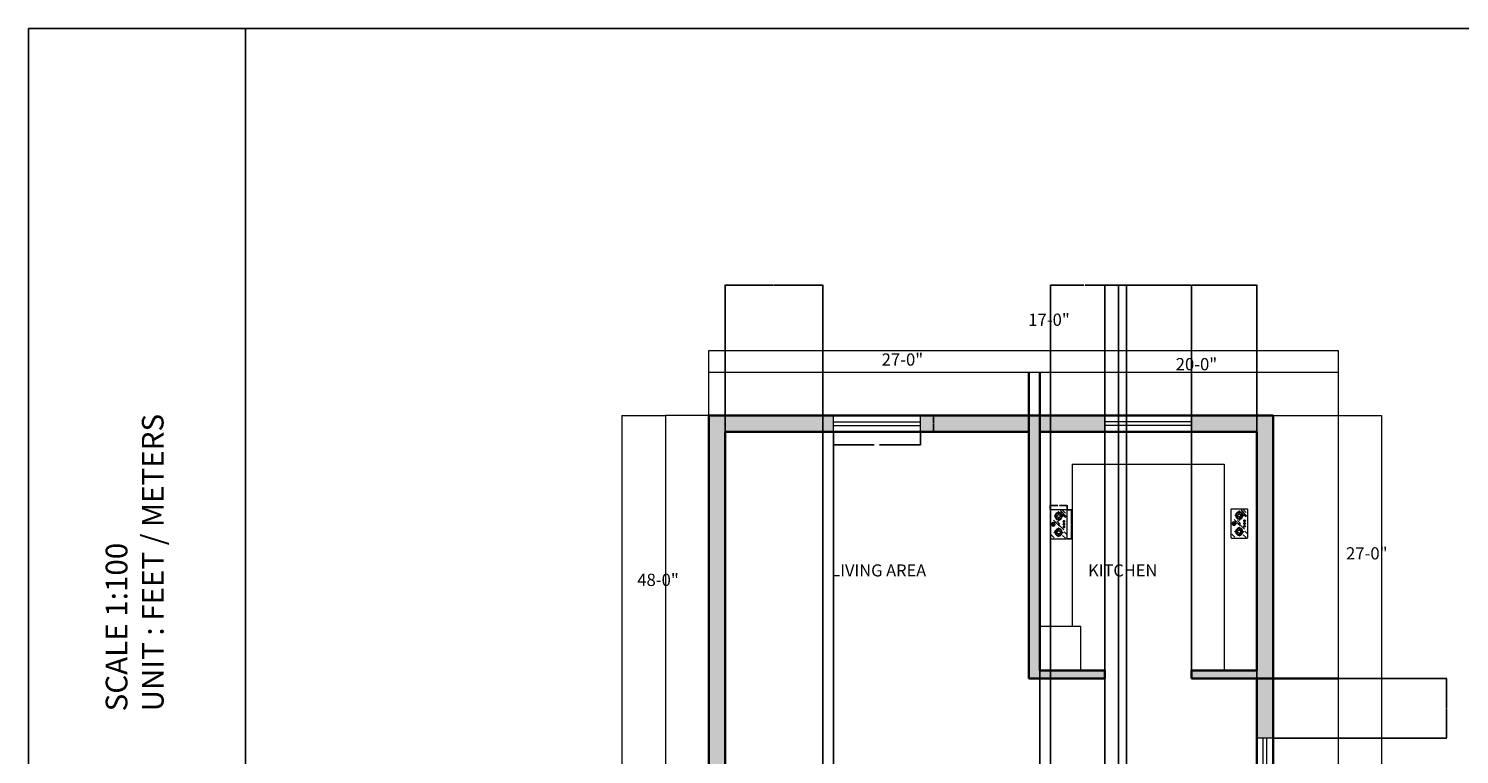
# Model space of a CAD drawing. Units: feet. Extents: x 2813 to 4435, y 1041 to 2557.
# Tile 3 of 6: x 2813 to 3605, y 2155 to 2557. Entities that reach past the tile are written whole.
import ezdxf

# ---------------------------------------------------------------- set-up
doc = ezdxf.new("R2010")
doc.units = ezdxf.units.FT
for name, color, linetype, lineweight in [('A-ANNO-DIMS', 2, 'Continuous', 18), ('A-ANNO-TTLB', 7, 'Continuous', 25), ('A-AREA-IDEN', 7, 'Continuous', 18), ('A-FLOR-CASE', 8, 'Continuous', 18), ('A-FLOR-FIXT', 9, 'Continuous', 18), ('A-GLAZ', 4, 'Continuous', 18), ('A-WALL', 7, 'Continuous', 35), ('A-WALL-PATT', 252, 'Continuous', 13)]:
    doc.layers.add(name, color=color, linetype=linetype, lineweight=lineweight)
doc.styles.get("Standard").update_dxf_attribs({"font": 'arial.ttf'})
doc.dimstyles.get("Standard").update_dxf_attribs({"dimtxt": 0.18, "dimasz": 0.18, "dimexe": 0.18, "dimexo": 0.0625, "dimgap": 0.09, "dimtad": 0, "dimtih": 1, "dimtoh": 1, "dimdec": 4, "dimzin": 0, "dimdsep": 46, "dimtxsty": 'Standard', "dimcen": 0.09, "dimadec": 0, "dimazin": 0, "dimtfac": 1, "dimtdec": 4, "dimtofl": 0, "dimtmove": 0, "dimatfit": 3, "dimfxl": 1, "dimtolj": 1, "dimtzin": 0, "dimarcsym": 0})

# ---------------------------------------------------------------- blocks, each defined once
blk = doc.blocks.new('A$C64847A4C')
for p, q in [((24, 337), (101, 414)), ((377, 411), (372, 411)), ((10, 41), (87, 118)), ((53, 225), (53, 220)), ((101, 2), (178, 79)), ((232, 89), (387, 244)), ((284, 225), (284, 220)), ((321, 203), (476, 357)), ((377, 306), (372, 306)), ((374, 194), (452, 271)), ((427, 360), (427, 355)), ((466, 225), (466, 220)), ((550, 48), (627, 125)), ((568, 22), (722, 177)), ((587, 340), (582, 340)), ((587, 104), (582, 104)), ((651, 92), (728, 170)), ((661, 42), (739, 119)), ((702, 225), (702, 220))]:
    blk.add_line(p, q)
at = {"ltscale": 0.18}
for p, q in [((372, 385), (372, 411)), ((377, 385), (377, 411)), ((120, 225), (53, 225)), ((120, 220), (53, 220)), ((163, 340), (168, 340)), ((163, 267), (163, 340)), ((163, 177), (163, 104)), ((163, 104), (168, 104)), ((168, 267), (168, 340)), ((168, 177), (168, 104)), ((210, 225), (284, 225)), ((210, 220), (284, 220)), ((299, 100), (299, 69)), ((307, 100), (307, 69)), ((348, 360), (322, 360)), ((322, 355), (322, 360)), ((348, 355), (322, 355)), ((372, 330), (372, 306)), ((372, 100), (372, 69)), ((377, 330), (377, 306)), ((380, 100), (380, 69)), ((402, 360), (427, 360)), ((402, 355), (427, 355)), ((443, 100), (443, 69)), ((451, 100), (451, 69)), ((540, 225), (466, 225)), ((540, 220), (466, 220)), ((582, 267), (582, 340)), ((582, 177), (582, 104)), ((587, 267), (587, 340)), ((587, 177), (587, 104)), ((630, 225), (702, 225)), ((630, 220), (702, 220))]:
    blk.add_line(p, q, dxfattribs=at)
blk.add_lwpolyline([(20, 0), (730, 0, 0.414214), (750, 20), (750, 420, 0.414214), (730, 440), (20, 440, 0.414214), (0, 420), (0, 20, 0.414214)], format="xyb", close=True)
for centre in [(346, 386), (89, 248), (95, 261), (509, 248), (515, 261)]:
    blk.add_circle(centre, 3.73)
for centre, radius in [((375, 357), 22.4), ((165, 222), 39), ((303, 84), 22.5), ((376, 84), 22.5), ((447, 84), 22.5), ((585, 222), 39)]:
    blk.add_circle(centre, radius, dxfattribs=at)
for centre, radius, start, end in [((375, 357), 47.4, 93.0255, 176.9745), ((375, 357), 37.4, 93.8363, 176.1637), ((375, 385), 2.52, 187.9505, 352.0495), ((375, 357), 47.4, 3.0255, 86.9745), ((375, 357), 37.4, 3.8363, 86.1637), ((165, 222), 95, 91.5918, 178.4082), ((165, 222), 95, 181.5918, 268.4082), ((165, 222), 75, 91.9102, 178.0898), ((165, 222), 75, 181.9102, 268.0898), ((119, 222), 2.64, 288.751, 71.249), ((165, 267), 2.52, 186.7354, 353.2646), ((165, 222), 95, 1.5918, 88.4082), ((165, 222), 75, 1.9102, 88.0898), ((165, 222), 95, 271.5918, 358.4082), ((165, 222), 75, 271.9102, 358.0898), ((211, 222), 2.67, 110.5507, 249.4493), ((303, 84), 18.5, 111.3237, 248.6763), ((297, 100), 2, 0, 111.3237), ((297, 69), 2, 248.6763, 0), ((309, 100), 2, 68.6763, 180), ((309, 69), 2, 180, 291.3237), ((303, 84), 18.5, 291.3237, 68.6763), ((375, 357), 47.4, 183.0255, 266.9745), ((375, 357), 37.4, 183.8363, 266.1637), ((347, 357), 2.62, 287.6318, 72.3682), ((376, 84), 18.5, 111.3237, 248.6763), ((370, 100), 2, 0, 111.3237), ((370, 69), 2, 248.6763, 0), ((375, 330), 2.5, 358.3317, 181.6683), ((375, 357), 37.4, 273.8363, 356.1637), ((375, 357), 47.4, 273.0255, 356.9745), ((382, 100), 2, 68.6763, 180), ((382, 69), 2, 180, 291.3237), ((376, 84), 18.5, 291.3237, 68.6763), ((403, 357), 2.52, 97.2236, 262.7764), ((447, 84), 18.5, 111.3237, 248.6763), ((441, 100), 2, 0, 111.3237), ((441, 69), 2, 248.6763, 0), ((453, 100), 2, 68.6763, 180), ((453, 69), 2, 180, 291.3237), ((447, 84), 18.5, 291.3237, 68.6763), ((585, 222), 95, 91.5918, 178.4082), ((585, 222), 95, 181.5918, 268.4082), ((585, 222), 75, 91.9102, 178.0898), ((585, 222), 75, 181.9102, 268.0898), ((539, 222), 2.63, 288.412, 71.588), ((585, 267), 2.51, 183.9579, 356.0421), ((585, 176), 2.63, 17.9418, 162.0582), ((585, 222), 75, 1.9102, 88.0898), ((585, 222), 75, 271.9102, 358.0898), ((585, 222), 95, 1.5918, 88.4082), ((585, 222), 95, 271.5918, 358.4082), ((630, 222), 2.58, 104.2945, 255.7055)]:
    blk.add_arc(centre, radius, start, end, dxfattribs=at)
blk.add_arc((165, 176), 2.69, 21.7885, 158.2115)
blk = doc.blocks.new('WINDOW-PLAN-WIDE')
for p, q in [((0, 0), (0, 9)), ((48, 0), (48, 9)), ((0, 5.5), (48, 5.5)), ((0, 3.5), (48, 3.5))]:
    blk.add_line(p, q)
blk = doc.blocks.new('*D19')
at = {"layer": 'A-ANNO-DIMS', "color": 0, "lineweight": -2, "transparency": 16777216}
for p, q in [((3258.56, 2333.52), (3258.56, 2326.2)), ((3258.74, 2326.38), (3281.08, 2326.38)), ((3306.38, 2326.38), (3284.04, 2326.38)), ((3306.56, 2333.52), (3306.56, 2326.2))]:
    blk.add_line(p, q, dxfattribs=at)
at = {"layer": 'A-ANNO-DIMS', "color": 0, "transparency": 16777216}
for points in [[(3258.74, 2326.41), (3258.74, 2326.35), (3258.56, 2326.38)], [(3306.38, 2326.41), (3306.38, 2326.35), (3306.56, 2326.38)]]:
    blk.add_solid(points, dxfattribs=at)
at = {"layer": 'DEFPOINTS', "color": 0, "transparency": 16777216}
for p in [(3258.56, 2333.58), (3306.56, 2333.58), (3306.56, 2326.38)]:
    blk.add_point(p, dxfattribs=at)
at = {"layer": 'A-ANNO-DIMS', "color": 0, "transparency": 16777216, "insert": (3282.56, 2326.38), "char_height": 0.18, "attachment_point": 5}
blk.add_mtext('\\A1;WIDE WINDOW 48 TYP.', dxfattribs=at)
blk = doc.blocks.new('*D20')
at = {"layer": 'A-ANNO-DIMS', "color": 0, "lineweight": -2, "transparency": 16777216}
for p, q in [((3306.62, 2342.58), (3313.94, 2342.58)), ((3313.76, 2342.4), (3313.76, 2338.26)), ((3313.76, 2333.76), (3313.76, 2337.9)), ((3306.62, 2333.58), (3313.94, 2333.58))]:
    blk.add_line(p, q, dxfattribs=at)
at = {"layer": 'A-ANNO-DIMS', "color": 0, "transparency": 16777216}
for points in [[(3313.73, 2342.4), (3313.79, 2342.4), (3313.76, 2342.58)], [(3313.73, 2333.76), (3313.79, 2333.76), (3313.76, 2333.58)]]:
    blk.add_solid(points, dxfattribs=at)
at = {"layer": 'DEFPOINTS', "color": 0, "transparency": 16777216}
for p in [(3306.56, 2342.58), (3313.76, 2342.58), (3306.56, 2333.58)]:
    blk.add_point(p, dxfattribs=at)
at = {"layer": 'A-ANNO-DIMS', "color": 0, "transparency": 16777216, "insert": (3313.76, 2338.08), "char_height": 0.18, "attachment_point": 5}
blk.add_mtext('\\A1;9 TYP.', dxfattribs=at)
blk = doc.blocks.new('*D27')
at = {"layer": 'A-ANNO-DIMS', "color": 0, "lineweight": -2, "transparency": 16777216}
for p, q in [((3387.82, 2290.44), (3390.34, 2290.44)), ((3390.16, 2290.26), (3390.16, 2282.61)), ((3390.16, 2274.6), (3390.16, 2282.24)), ((3387.82, 2274.42), (3390.34, 2274.42))]:
    blk.add_line(p, q, dxfattribs=at)
at = {"layer": 'A-ANNO-DIMS', "color": 0, "transparency": 16777216}
for points in [[(3390.13, 2290.26), (3390.19, 2290.26), (3390.16, 2290.44)], [(3390.13, 2274.6), (3390.19, 2274.6), (3390.16, 2274.42)]]:
    blk.add_solid(points, dxfattribs=at)
at = {"layer": 'DEFPOINTS', "color": 0, "transparency": 16777216}
for p in [(3387.75, 2290.44), (3390.16, 2290.44), (3387.75, 2274.42)]:
    blk.add_point(p, dxfattribs=at)
at = {"layer": 'A-ANNO-DIMS', "color": 0, "transparency": 16777216, "insert": (3390.16, 2282.43), "char_height": 0.18, "attachment_point": 5}
blk.add_mtext('\\A1;HOB 16 TYP.', dxfattribs=at)
blk = doc.blocks.new('*D28')
at = {"layer": 'A-ANNO-DIMS', "color": 0, "lineweight": -2, "transparency": 16777216}
for p, q in [((3378.36, 2290.5), (3378.36, 2293.02)), ((3378.54, 2292.84), (3382.6, 2292.84)), ((3387.57, 2292.84), (3383.51, 2292.84)), ((3387.75, 2290.5), (3387.75, 2293.02))]:
    blk.add_line(p, q, dxfattribs=at)
at = {"layer": 'A-ANNO-DIMS', "color": 0, "transparency": 16777216}
for points in [[(3378.54, 2292.87), (3378.54, 2292.81), (3378.36, 2292.84)], [(3387.57, 2292.87), (3387.57, 2292.81), (3387.75, 2292.84)]]:
    blk.add_solid(points, dxfattribs=at)
at = {"layer": 'DEFPOINTS', "color": 0, "transparency": 16777216}
for p in [(3378.36, 2292.84), (3378.36, 2290.44), (3387.75, 2290.44)]:
    blk.add_point(p, dxfattribs=at)
at = {"layer": 'A-ANNO-DIMS', "color": 0, "transparency": 16777216, "insert": (3383.06, 2292.84), "char_height": 0.18, "attachment_point": 5}
blk.add_mtext('\\A1;9 TYP.', dxfattribs=at)
blk = doc.blocks.new('*D52')
at = {"layer": 'A-ANNO-DIMS', "color": 0, "lineweight": -2, "transparency": 16777216}
for p, q in [((3198.56, 2333.52), (3198.56, 1691.4)), ((3258.56, 2333.52), (3258.56, 1691.4)), ((3198.74, 1691.58), (3228.34, 1691.58)), ((3258.38, 1691.58), (3228.78, 1691.58))]:
    blk.add_line(p, q, dxfattribs=at)
at = {"layer": 'A-ANNO-DIMS', "color": 0, "transparency": 16777216}
for points in [[(3198.74, 1691.61), (3198.74, 1691.55), (3198.56, 1691.58)], [(3258.38, 1691.61), (3258.38, 1691.55), (3258.56, 1691.58)]]:
    blk.add_solid(points, dxfattribs=at)
at = {"layer": 'DEFPOINTS', "color": 0, "transparency": 16777216}
for p in [(3198.56, 2333.58), (3258.56, 2333.58), (3258.56, 1691.58)]:
    blk.add_point(p, dxfattribs=at)
at = {"layer": 'A-ANNO-DIMS', "color": 0, "transparency": 16777216, "insert": (3228.56, 1691.58), "char_height": 0.18, "attachment_point": 5}
blk.add_mtext('\\A1;60', dxfattribs=at)
blk = doc.blocks.new('*D53')
at = {"layer": 'A-ANNO-DIMS', "color": 0, "lineweight": -2, "transparency": 16777216}
for p, q in [((3372.56, 2333.52), (3372.56, 1691.4)), ((3408.56, 2333.52), (3408.56, 1691.4)), ((3372.74, 1691.58), (3390.34, 1691.58)), ((3408.38, 1691.58), (3390.78, 1691.58))]:
    blk.add_line(p, q, dxfattribs=at)
at = {"layer": 'A-ANNO-DIMS', "color": 0, "transparency": 16777216}
for points in [[(3372.74, 1691.61), (3372.74, 1691.55), (3372.56, 1691.58)], [(3408.38, 1691.61), (3408.38, 1691.55), (3408.56, 1691.58)]]:
    blk.add_solid(points, dxfattribs=at)
at = {"layer": 'DEFPOINTS', "color": 0, "transparency": 16777216}
for p in [(3372.56, 2333.58), (3408.56, 2333.58), (3408.56, 1691.58)]:
    blk.add_point(p, dxfattribs=at)
at = {"layer": 'A-ANNO-DIMS', "color": 0, "transparency": 16777216, "insert": (3390.56, 1691.58), "char_height": 0.18, "attachment_point": 5}
blk.add_mtext('\\A1;36', dxfattribs=at)
blk = doc.blocks.new('*D54')
at = {"layer": 'A-ANNO-DIMS', "color": 0, "lineweight": -2, "transparency": 16777216}
for p, q in [((3408.56, 2197.15), (3408.56, 2414.76)), ((3408.74, 2414.58), (3432.33, 2414.58)), ((3456.38, 2414.58), (3432.78, 2414.58)), ((3456.56, 2197.15), (3456.56, 2414.76))]:
    blk.add_line(p, q, dxfattribs=at)
at = {"layer": 'A-ANNO-DIMS', "color": 0, "transparency": 16777216}
for points in [[(3408.74, 2414.61), (3408.74, 2414.55), (3408.56, 2414.58)], [(3456.38, 2414.61), (3456.38, 2414.55), (3456.56, 2414.58)]]:
    blk.add_solid(points, dxfattribs=at)
at = {"layer": 'DEFPOINTS', "color": 0, "transparency": 16777216}
for p in [(3456.56, 2414.58), (3408.56, 2197.08), (3456.56, 2197.08)]:
    blk.add_point(p, dxfattribs=at)
at = {"layer": 'A-ANNO-DIMS', "color": 0, "transparency": 16777216, "insert": (3432.56, 2414.58), "char_height": 0.18, "attachment_point": 5}
blk.add_mtext('\\A1;48', dxfattribs=at)
blk = doc.blocks.new('*D57')
at = {"layer": 'A-ANNO-DIMS', "color": 0, "lineweight": -2, "transparency": 16777216}
for p, q in [((3198.56, 1889.65), (3198.56, 2414.76)), ((3198.74, 2414.58), (3225.34, 2414.58)), ((3252.38, 2414.58), (3225.78, 2414.58)), ((3252.56, 1889.65), (3252.56, 2414.76))]:
    blk.add_line(p, q, dxfattribs=at)
at = {"layer": 'A-ANNO-DIMS', "color": 0, "transparency": 16777216}
for points in [[(3198.74, 2414.61), (3198.74, 2414.55), (3198.56, 2414.58)], [(3252.38, 2414.61), (3252.38, 2414.55), (3252.56, 2414.58)]]:
    blk.add_solid(points, dxfattribs=at)
at = {"layer": 'DEFPOINTS', "color": 0, "transparency": 16777216}
for p in [(3198.56, 2414.58), (3198.56, 1889.58), (3252.56, 1889.58)]:
    blk.add_point(p, dxfattribs=at)
at = {"layer": 'A-ANNO-DIMS', "color": 0, "transparency": 16777216, "insert": (3225.56, 2414.58), "char_height": 0.18, "attachment_point": 5}
blk.add_mtext('\\A1;54', dxfattribs=at)
blk = doc.blocks.new('*D59')
at = {"layer": 'A-ANNO-DIMS', "color": 0, "lineweight": -2, "transparency": 16777216}
for p, q in [((3420.56, 1991.65), (3420.56, 2414.76)), ((3420.74, 2414.58), (3456.34, 2414.58)), ((3492.38, 2414.58), (3456.77, 2414.58)), ((3492.56, 1991.65), (3492.56, 2414.76))]:
    blk.add_line(p, q, dxfattribs=at)
at = {"layer": 'A-ANNO-DIMS', "color": 0, "transparency": 16777216}
for points in [[(3420.74, 2414.61), (3420.74, 2414.55), (3420.56, 2414.58)], [(3492.38, 2414.61), (3492.38, 2414.55), (3492.56, 2414.58)]]:
    blk.add_solid(points, dxfattribs=at)
at = {"layer": 'DEFPOINTS', "color": 0, "transparency": 16777216}
for p in [(3492.56, 2414.58), (3420.56, 1991.58), (3492.56, 1991.58)]:
    blk.add_point(p, dxfattribs=at)
at = {"layer": 'A-ANNO-DIMS', "color": 0, "transparency": 16777216, "insert": (3456.56, 2414.58), "char_height": 0.18, "attachment_point": 5}
blk.add_mtext('\\A1;72', dxfattribs=at)
blk = doc.blocks.new('*D72')
at = {"layer": 'A-ANNO-DIMS', "color": 0, "lineweight": -2, "transparency": 16777216}
for p, q in [((3378.56, 1991.65), (3378.56, 2414.76)), ((3378.74, 2414.58), (3396.98, 2414.58)), ((3415.88, 2414.58), (3397.63, 2414.58)), ((3416.06, 1987.15), (3416.06, 2414.76))]:
    blk.add_line(p, q, dxfattribs=at)
at = {"layer": 'A-ANNO-DIMS', "color": 0, "transparency": 16777216}
for points in [[(3378.74, 2414.61), (3378.74, 2414.55), (3378.56, 2414.58)], [(3415.88, 2414.61), (3415.88, 2414.55), (3416.06, 2414.58)]]:
    blk.add_solid(points, dxfattribs=at)
at = {"layer": 'DEFPOINTS', "color": 0, "transparency": 16777216}
for p in [(3416.06, 2414.58), (3378.56, 1991.58), (3416.06, 1987.08)]:
    blk.add_point(p, dxfattribs=at)
at = {"layer": 'A-ANNO-DIMS', "color": 0, "transparency": 16777216, "insert": (3397.31, 2414.58), "char_height": 0.18, "attachment_point": 5}
blk.add_mtext('\\A1;37.5', dxfattribs=at)
blk = doc.blocks.new('*D74')
at = {"layer": 'A-ANNO-DIMS', "color": 0, "lineweight": -2, "transparency": 16777216}
for p, q in [((3492.62, 2197.08), (3597.74, 2197.08)), ((3597.56, 2196.9), (3597.56, 2180.76)), ((3597.56, 2164.26), (3597.56, 2180.4)), ((3501.62, 2164.08), (3597.74, 2164.08))]:
    blk.add_line(p, q, dxfattribs=at)
at = {"layer": 'A-ANNO-DIMS', "color": 0, "transparency": 16777216}
for points in [[(3597.53, 2196.9), (3597.59, 2196.9), (3597.56, 2197.08)], [(3597.53, 2164.26), (3597.59, 2164.26), (3597.56, 2164.08)]]:
    blk.add_solid(points, dxfattribs=at)
at = {"layer": 'DEFPOINTS', "color": 0, "transparency": 16777216}
for p in [(3492.56, 2197.08), (3501.56, 2164.08), (3597.56, 2164.08)]:
    blk.add_point(p, dxfattribs=at)
at = {"layer": 'A-ANNO-DIMS', "color": 0, "transparency": 16777216, "insert": (3597.56, 2180.58), "char_height": 0.18, "attachment_point": 5}
blk.add_mtext('\\A1;33', dxfattribs=at)

msp = doc.modelspace()

# ---------------------------------------------------------------- hatches: boundary and pattern name
at = {"layer": 'A-WALL-PATT'}
h = msp.add_hatch(color=256, dxfattribs=at)
h.dxf.hatch_style = 1
h.paths.add_polyline_path([(3198.557, 2333.583), (3258.557, 2333.583), (3258.557, 2342.583), (3189.557, 2342.583), (3189.557, 2135.583), (3372.557, 2135.583), (3372.557, 2141.583), (3198.557, 2141.583)])
h.paths.add_polyline_path([(3366.557, 2342.583), (3306.557, 2342.583), (3306.557, 2333.583), (3366.557, 2333.583)], flags=17)
h.paths.add_polyline_path([(3372.557, 2342.583), (3366.557, 2342.583), (3366.557, 2197.083), (3372.557, 2197.083), (3408.557, 2197.083), (3408.557, 2201.583), (3372.557, 2201.583), (3372.557, 2225.773)])
h.paths.add_polyline_path([(3408.557, 2342.583), (3372.557, 2342.583), (3372.557, 2333.583), (3408.557, 2333.583)], flags=17)
h.paths.add_polyline_path([(3501.557, 2342.583), (3456.557, 2342.583), (3456.557, 2333.583), (3492.557, 2333.583), (3492.557, 2201.583), (3456.557, 2201.583), (3456.557, 2197.083), (3501.557, 2197.083)])
h.paths.add_polyline_path([(3501.557, 2197.083), (3492.557, 2197.083), (3492.557, 2164.083), (3501.557, 2164.083)])
h.paths.add_polyline_path([(3501.557, 2116.083), (3492.557, 2116.083), (3492.557, 2083.083), (3420.557, 2083.083), (3420.557, 2077.083), (3501.557, 2077.083)])
h.paths.add_polyline_path([(3501.557, 2077.083), (3492.557, 2077.083), (3492.557, 2046.333), (3501.557, 2046.333)])
h.paths.add_polyline_path([(3501.557, 2022.333), (3492.557, 2022.333), (3492.557, 1991.583), (3420.557, 1991.583), (3420.557, 1987.083), (3492.557, 1987.083), (3492.557, 1843.083), (3456.557, 1843.083), (3456.557, 1834.083), (3501.557, 1834.083)])
h.paths.add_polyline_path([(3408.557, 1843.083), (3372.557, 1843.083), (3372.557, 1834.083), (3408.557, 1834.083)])
h.paths.add_polyline_path([(3372.557, 1987.083), (3378.557, 1987.083), (3378.557, 1991.583), (3372.557, 1991.583), (3366.557, 1991.583), (3366.557, 1889.583), (3360.557, 1889.583), (3360.557, 1883.583), (3366.557, 1883.583), (3366.557, 1763.583), (3372.557, 1763.583)])
h.paths.add_polyline_path([(3198.557, 1883.583), (3189.557, 1883.583), (3189.557, 1763.583), (3198.557, 1763.583)])
h.paths.add_polyline_path([(3198.557, 2033.583), (3234.557, 2033.583), (3234.557, 2039.583), (3189.557, 2039.583), (3189.557, 1883.583), (3198.557, 1883.583), (3252.557, 1883.583), (3252.557, 1889.583), (3198.557, 1889.583)])
h.paths.add_polyline_path([(3198.557, 2063.583), (3189.557, 2063.583), (3189.557, 2039.583), (3198.557, 2039.583)])
h.paths.add_polyline_path([(3198.557, 2135.583), (3189.557, 2135.583), (3189.557, 2111.583), (3198.557, 2111.583)])
h.paths.add_polyline_path([(3312.557, 1889.583), (3300.557, 1889.583), (3300.557, 1883.583), (3312.557, 1883.583)])

# ---------------------------------------------------------------- linework, layer by layer
at = {"layer": 'A-ANNO-DIMS'}
for p, q in [((3189.557, 2111.583), (3189.557, 2378.583)), ((3189.557, 2378.583), (3537.557, 2378.583)), ((3537.557, 2378.583), (3537.557, 2197.083)), ((3189.557, 2366.583), (3537.557, 2366.583)), ((3141.557, 2342.583), (3141.557, 1763.583)), ((3141.557, 2342.583), (3165.557, 2342.583)), ((3189.557, 2342.583), (3165.557, 2342.583)), ((3165.557, 2342.583), (3165.557, 1763.583)), ((3501.557, 2342.583), (3537.557, 2342.583)), ((3537.557, 2342.583), (3537.557, 1834.083)), ((3537.557, 2342.583), (3561.557, 2342.583)), ((3561.557, 2342.583), (3561.557, 1834.083))]:
    msp.add_line(p, q, dxfattribs=at)
at = {"layer": 'A-ANNO-TTLB'}
for p, q in [((2813.466, 1041.465), (2813.466, 2556.562)), ((2813.466, 2556.562), (2933.466, 2556.562)), ((2933.466, 2556.562), (4435.474, 2556.562)), ((2933.466, 1041.465), (2933.466, 2556.562))]:
    msp.add_line(p, q, dxfattribs=at)
at = {"layer": 'A-FLOR-CASE'}
for p, q in [((3390.557, 2315.583), (3390.557, 2225.773)), ((3390.557, 2315.583), (3474.557, 2315.583)), ((3474.557, 2315.583), (3474.557, 2201.583))]:
    msp.add_line(p, q, dxfattribs=at)
msp.add_lwpolyline([(3372.557, 2201.583), (3395.31, 2201.583), (3395.31, 2225.773), (3372.557, 2225.773)], close=True, dxfattribs=at)
at = {"layer": 'A-WALL'}
for p, q in [((3366.557, 2366.583), (3366.557, 2197.083)), ((3372.557, 2366.583), (3372.557, 2201.583)), ((3189.557, 2342.583), (3501.557, 2342.583)), ((3189.557, 2342.583), (3189.557, 1763.583)), ((3501.557, 2342.583), (3501.557, 1834.083)), ((3198.557, 2333.583), (3366.557, 2333.583)), ((3198.557, 2333.583), (3198.557, 2141.583)), ((3372.557, 2333.583), (3492.557, 2333.583)), ((3492.557, 2333.583), (3492.557, 2201.583)), ((3372.557, 2201.583), (3408.557, 2201.583)), ((3408.557, 2201.583), (3408.557, 2197.083)), ((3456.557, 2201.583), (3492.557, 2201.583)), ((3456.557, 2201.583), (3456.557, 2197.083)), ((3372.557, 2197.083), (3366.557, 2197.083)), ((3372.557, 2197.083), (3408.557, 2197.083)), ((3456.557, 2197.083), (3537.557, 2197.083)), ((3492.557, 2197.083), (3492.557, 2083.083))]:
    msp.add_line(p, q, dxfattribs=at)

# ---------------------------------------------------------------- block references
at = {"layer": 'A-FLOR-FIXT', "xscale": 0.0213579260599023, "yscale": 0.0213579260599023, "zscale": 0.0213579260599023, "rotation": 90}
for p in [(3387.755, 2274.418), (3487.634, 2274.778)]:
    msp.add_blockref('A$C64847A4C', p, dxfattribs=at)
at = {"layer": 'A-GLAZ'}
msp.add_blockref('WINDOW-PLAN-WIDE', (3258.557, 2333.583), dxfattribs=at)
for p, rotation in [((3456.557, 2342.582), 180), ((3501.557, 2116.083), 90.00000000000063)]:
    msp.add_blockref('WINDOW-PLAN-WIDE', p, dxfattribs=dict(at, rotation=rotation))

# ---------------------------------------------------------------- texts
at = {"layer": 'A-ANNO-DIMS', "char_height": 6.7726, "attachment_point": 1}
for s, insert in [('17-0" ', (3366.209, 2398.926)), ('27-0" ', (3285.147, 2376.906)), ('20-0" ', (3447.737, 2374.338)), ('27-0" ', (3541.928, 2269.694)), ('48-0" ', (3150.003, 2255.039))]:
    msp.add_mtext_dynamic_manual_height_columns(s, width=22.46964, gutter_width=33.863, heights=[0], dxfattribs=dict(at, insert=insert))
at = {"layer": 'A-ANNO-TTLB', "insert": (2856.091, 2178.904), "char_height": 12, "attachment_point": 1, "rotation": 90}
msp.add_mtext_dynamic_manual_height_columns('SCALE 1:100\\PUNIT : FEET / METERS', width=375.25864, gutter_width=7.02, heights=[0], dxfattribs=at)
at = {"layer": 'A-AREA-IDEN', "attachment_point": 1}
for s, insert, char_height in [('LIVING AREA', (3257.32, 2260.195), 6.65198), ('KITCHEN', (3399.33, 2260.195), 6.652)]:
    msp.add_mtext_dynamic_manual_height_columns(s, width=109.65837, gutter_width=33.26, heights=[0], dxfattribs=dict(at, insert=insert, char_height=char_height))

# ---------------------------------------------------------------- dimensions: what is measured, and where the dimension line sits
at = {"layer": 'A-ANNO-DIMS'}
for base, p1, p2, override, picture, middle in [((3198.557, 2414.583), (3252.557, 1889.583), (3198.557, 1889.583), {"dimdec": 0, "dimlfac": 1, "dimrnd": 0, "dimzin": 0, "dimdsep": 46, "dimlunit": 2}, '*D57', (3225.557, 2414.583)), ((3416.057, 2414.583), (3378.557, 1991.583), (3416.057, 1987.083), {"dimdec": 1, "dimlfac": 1, "dimrnd": 0, "dimzin": 0, "dimdsep": 46, "dimlunit": 2}, '*D72', (3397.307, 2414.583)), ((3456.557, 2414.583), (3408.557, 2197.083), (3456.557, 2197.083), {"dimdec": 0, "dimlfac": 1, "dimrnd": 0, "dimzin": 0, "dimdsep": 46, "dimlunit": 2}, '*D54', (3432.557, 2414.583)), ((3492.557, 2414.583), (3420.557, 1991.583), (3492.557, 1991.583), {"dimdec": 0, "dimlfac": 1, "dimrnd": 0, "dimzin": 0, "dimdsep": 46, "dimlunit": 2}, '*D59', (3456.557, 2414.583)), ((3258.557, 1691.583), (3198.557, 2333.583), (3258.557, 2333.583), {"dimdec": 0, "dimlfac": 1, "dimrnd": 0, "dimzin": 0, "dimdsep": 46, "dimlunit": 2}, '*D52', (3228.557, 1691.583)), ((3408.557, 1691.583), (3372.557, 2333.583), (3408.557, 2333.583), {"dimdec": 0, "dimlfac": 1, "dimrnd": 0, "dimzin": 0, "dimdsep": 46, "dimlunit": 2}, '*D53', (3390.557, 1691.583))]:
    dim = msp.add_linear_dim(base=base, p1=p1, p2=p2, dimstyle='Standard', override=override, dxfattribs=at)
    dim.commit()
    dim.dimension.update_dxf_attribs({"geometry": picture, "text_midpoint": middle})
for base, p1, p2, angle, text, picture, middle in [((3313.757, 2342.583), (3306.557, 2333.583), (3306.557, 2342.583), 90, '<> TYP.', '*D20', (3313.757, 2338.083)), ((3378.357, 2292.839), (3387.755, 2290.437), (3378.357, 2290.437), 180, '<> TYP.', '*D28', (3383.056, 2292.839)), ((3390.157, 2290.437), (3387.755, 2274.418), (3387.755, 2290.437), 90, 'HOB <> TYP.', '*D27', (3390.157, 2282.427))]:
    dim = msp.add_linear_dim(base=base, p1=p1, p2=p2, angle=angle, text=text, dimstyle='Standard', override={"dimdec": 0, "dimlfac": 1, "dimrnd": 0, "dimzin": 0, "dimdsep": 46, "dimlunit": 2}, dxfattribs=at)
    dim.commit()
    dim.dimension.update_dxf_attribs({"geometry": picture, "text_midpoint": middle})
dim = msp.add_linear_dim(base=(3306.557, 2326.383), p1=(3258.557, 2333.583), p2=(3306.557, 2333.583), text='WIDE WINDOW <> TYP.', dimstyle='Standard', override={"dimdec": 0, "dimlfac": 1, "dimrnd": 0, "dimzin": 0, "dimdsep": 46, "dimlunit": 2}, dxfattribs=at)
dim.commit()
dim.dimension.update_dxf_attribs({"geometry": '*D19', "text_midpoint": (3282.557, 2326.383)})
dim = msp.add_linear_dim(base=(3597.557, 2164.083), p1=(3492.557, 2197.083), p2=(3501.557, 2164.083), angle=90, dimstyle='Standard', override={"dimdec": 0, "dimlfac": 1, "dimrnd": 0, "dimzin": 0, "dimdsep": 46, "dimlunit": 2}, dxfattribs=at)
dim.commit()
dim.dimension.update_dxf_attribs({"geometry": '*D74', "text_midpoint": (3597.557, 2180.583)})

doc.saveas('drawing.dxf')
